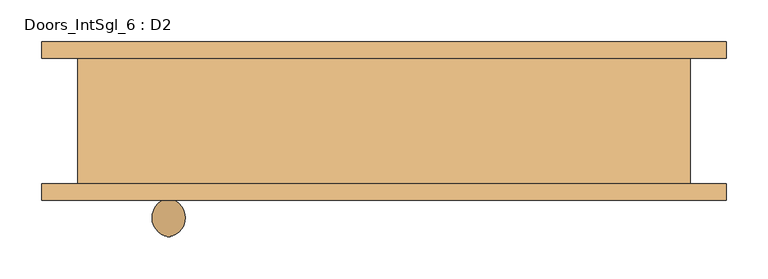
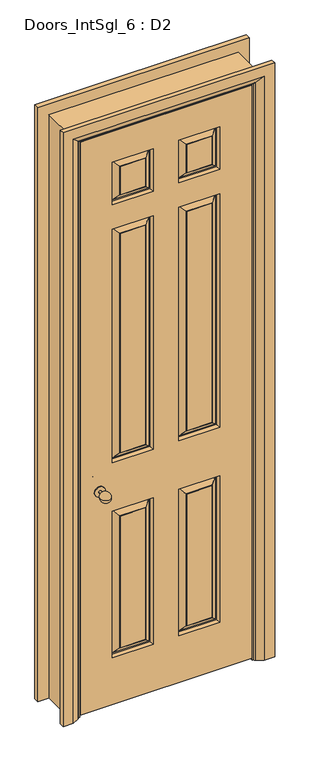
"""IFC4 building model written with IfcOpenShell, lengths in millimetres: door geometry, Doors_IntSgl_6 : D2."""

from ifc_helpers import new_model, si_unit, point, frame, origin, place, context, project, spatial, polyline, circle_curve, ellipse_curve, trimmed, outline, extrude, faceted_brep, source, transform, mapped, element, save
from ifc_brep_helpers import plane_surface, cylinder_surface, revolved_surface, advanced_brep


def doors_intsgl_6_d2_ad12cddb(model_context):
    return source(origin(), model_context, "Body", "SolidModel", [
        advanced_brep(
        [(-253.0, -18.0, 900.0), (-263.0, -18.0, 900.0), (-258.0, 26.437411, 900.0), (-253.0, -33.0, 900.0), (-263.0, -33.0, 900.0), (-278.0, -37.0, 900.0), (-238.0, -37.0, 900.0), (-278.0, -33.0, 900.0), (-238.0, -33.0, 900.0)],
        [
            (0, 1, circle_curve(frame((-258.0, -18.0, 900.0), z_axis=(0.0, 1.0, 0.0), x_axis=(-1.0, 0.0, 0.0)), 5.0)),
            (1, 2, circle_curve(frame((-254.8115138, 3.5786495, 900.0), z_axis=(0.0, 0.0, -1.0), x_axis=(0.0, -1.0, 0.0)), 23.0800654)),
            (2, 0, circle_curve(frame((-261.1884862, 3.5786495, 900.0), z_axis=(0.0, 0.0, -1.0), x_axis=(0.0, -1.0, 0.0)), 23.0800654)),
            (1, 0, circle_curve(frame((-258.0, -18.0, 900.0), z_axis=(0.0, 1.0, 0.0), x_axis=(-1.0, 0.0, 0.0)), 5.0)),
            (0, 3),
            (3, 4, circle_curve(frame((-258.0, -33.0, 900.0), z_axis=(0.0, 1.0, 0.0), x_axis=(-1.0, 0.0, 0.0)), 5.0)),
            (4, 1),
            (4, 3, circle_curve(frame((-258.0, -33.0, 900.0), z_axis=(0.0, 1.0, 0.0), x_axis=(-1.0, 0.0, 0.0)), 5.0)),
            (5, 6, circle_curve(frame((-258.0, -37.0, 900.0), z_axis=(0.0, -1.0, 0.0), x_axis=(1.0, 0.0, 0.0)), 20.0)),
            (6, 5, circle_curve(frame((-258.0, -37.0, 900.0), z_axis=(0.0, -1.0, 0.0), x_axis=(1.0, 0.0, 0.0)), 20.0)),
            (7, 8, circle_curve(frame((-258.0, -33.0, 900.0), z_axis=(0.0, 1.0, 0.0), x_axis=(1.0, 0.0, 0.0)), 20.0)),
            (8, 7, circle_curve(frame((-258.0, -33.0, 900.0), z_axis=(0.0, 1.0, 0.0), x_axis=(1.0, 0.0, 0.0)), 20.0)),
            (5, 7),
            (8, 6),
        ],
        [
            revolved_surface(trimmed(ellipse_curve(frame((-254.8115138, 3.5786495, 900.0), z_axis=(0.0, 0.0, 1.0), x_axis=(0.0, -1.0, 0.0)), 23.0800654, 23.0800654), [point((-258.0, 26.437411, 900.0))], [point((-263.0, -18.0, 900.0))], True, "CARTESIAN"), (-258.0, -33.0, 900.0), (0.0, -1.0, 0.0)),
            cylinder_surface(frame((-258.0, -33.0, 900.0), z_axis=(0.0, -1.0, 0.0), x_axis=(-1.0, 0.0, 0.0)), 5.0),
            plane_surface(frame((-238.0, -37.0, 900.0), z_axis=(0.0, -1.0, 0.0), x_axis=(0.0, 0.0, 1.0))),
            plane_surface(frame((-238.0, -33.0, 900.0), z_axis=(0.0, 1.0, 0.0), x_axis=(0.0, 0.0, -1.0))),
            cylinder_surface(frame((-258.0, -33.0, 900.0), z_axis=(0.0, -1.0, 0.0), x_axis=(1.0, 0.0, 0.0)), 20.0),
        ],
        [
            (0, [[1, 2, 3]]),
            (0, [[-2, 4, -3]]),
            (1, [[-1, 5, 6, 7]]),
            (1, [[-4, -7, 8, -5]]),
            (2, [[9, 10]]),
            (3, [[11, 12], [-6, -8]]),
            (4, [[-9, 13, -12, 14]]),
            (4, [[-10, -14, -11, -13]]),
        ],
    ),
        advanced_brep(
        [(-253.0, -94.0, 900.0), (-258.0, -138.437411, 900.0), (-263.0, -94.0, 900.0), (-263.0, -79.0, 900.0), (-253.0, -79.0, 900.0), (-278.0, -75.0, 900.0), (-238.0, -75.0, 900.0), (-278.0, -79.0, 900.0), (-238.0, -79.0, 900.0)],
        [
            (0, 1, circle_curve(frame((-261.1884862, -115.5786495, 900.0), z_axis=(0.0, 0.0, -1.0), x_axis=(0.0, 1.0, 0.0)), 23.0800654)),
            (1, 2, circle_curve(frame((-254.8115138, -115.5786495, 900.0), z_axis=(0.0, 0.0, -1.0), x_axis=(0.0, 1.0, 0.0)), 23.0800654)),
            (2, 0, circle_curve(frame((-258.0, -94.0, 900.0), z_axis=(0.0, -1.0, 0.0), x_axis=(-1.0, 0.0, 0.0)), 5.0)),
            (0, 2, circle_curve(frame((-258.0, -94.0, 900.0), z_axis=(0.0, -1.0, 0.0), x_axis=(-1.0, 0.0, 0.0)), 5.0)),
            (2, 3),
            (3, 4, circle_curve(frame((-258.0, -79.0, 900.0), z_axis=(0.0, -1.0, 0.0), x_axis=(-1.0, 0.0, 0.0)), 5.0)),
            (4, 0),
            (4, 3, circle_curve(frame((-258.0, -79.0, 900.0), z_axis=(0.0, -1.0, 0.0), x_axis=(-1.0, 0.0, 0.0)), 5.0)),
            (5, 6, circle_curve(frame((-258.0, -75.0, 900.0), z_axis=(0.0, 1.0, 0.0), x_axis=(1.0, 0.0, 0.0)), 20.0)),
            (6, 5, circle_curve(frame((-258.0, -75.0, 900.0), z_axis=(0.0, 1.0, 0.0), x_axis=(1.0, 0.0, 0.0)), 20.0)),
            (7, 8, circle_curve(frame((-258.0, -79.0, 900.0), z_axis=(0.0, -1.0, 0.0), x_axis=(1.0, 0.0, 0.0)), 20.0)),
            (8, 7, circle_curve(frame((-258.0, -79.0, 900.0), z_axis=(0.0, -1.0, 0.0), x_axis=(1.0, 0.0, 0.0)), 20.0)),
            (6, 8),
            (7, 5),
        ],
        [
            revolved_surface(trimmed(ellipse_curve(frame((-254.8115138, -115.5786495, 900.0), z_axis=(0.0, 0.0, -1.0), x_axis=(0.0, 1.0, 0.0)), 23.0800654, 23.0800654), [point((-258.0, -138.437411, 900.0))], [point((-263.0, -94.0, 900.0))], True, "CARTESIAN"), (-258.0, -79.0, 900.0), (0.0, 1.0, 0.0)),
            cylinder_surface(frame((-258.0, -79.0, 900.0), z_axis=(0.0, 1.0, 0.0), x_axis=(-1.0, 0.0, 0.0)), 5.0),
            plane_surface(frame((-238.0, -75.0, 900.0), z_axis=(0.0, 1.0, 0.0), x_axis=(0.0, 0.0, 1.0))),
            plane_surface(frame((-238.0, -79.0, 900.0), z_axis=(0.0, -1.0, 0.0), x_axis=(0.0, 0.0, -1.0))),
            cylinder_surface(frame((-258.0, -79.0, 900.0), z_axis=(0.0, 1.0, 0.0), x_axis=(1.0, 0.0, 0.0)), 20.0),
        ],
        [
            (0, [[1, 2, 3]]),
            (0, [[-1, 4, -2]]),
            (1, [[5, 6, 7, -3]]),
            (1, [[-7, 8, -5, -4]]),
            (2, [[9, 10]]),
            (3, [[11, 12], [-8, -6]]),
            (4, [[13, -11, 14, -10]]),
            (4, [[-14, -12, -13, -9]]),
        ],
    ),
        faceted_brep([(-333.0, -37.0, 2358.0), (333.0, -37.0, 2358.0), (333.0, -37.0, 8.0), (-333.0, -37.0, 8.0), (-50.0, -37.0, 800.0), (-208.0, -37.0, 800.0), (-208.0, -37.0, 200.0), (-50.0, -37.0, 200.0), (208.0, -37.0, 800.0), (50.0, -37.0, 800.0), (50.0, -37.0, 200.0), (208.0, -37.0, 200.0), (-50.0, -37.0, 1958.0), (-208.0, -37.0, 1958.0), (-208.0, -37.0, 1000.0), (-50.0, -37.0, 1000.0), (208.0, -37.0, 1958.0), (50.0, -37.0, 1958.0), (50.0, -37.0, 1000.0), (208.0, -37.0, 1000.0), (-50.0, -37.0, 2233.0), (-208.0, -37.0, 2233.0), (-208.0, -37.0, 2058.0), (-50.0, -37.0, 2058.0), (208.0, -37.0, 2233.0), (50.0, -37.0, 2233.0), (50.0, -37.0, 2058.0), (208.0, -37.0, 2058.0), (-80.0, -37.0, 230.0), (-178.0, -37.0, 230.0), (-178.0, -37.0, 770.0), (-80.0, -37.0, 770.0), (178.0, -37.0, 230.0), (80.0, -37.0, 230.0), (80.0, -37.0, 770.0), (178.0, -37.0, 770.0), (-80.0, -37.0, 1030.0), (-178.0, -37.0, 1030.0), (-178.0, -37.0, 1928.0), (-80.0, -37.0, 1928.0), (178.0, -37.0, 1030.0), (80.0, -37.0, 1030.0), (80.0, -37.0, 1928.0), (178.0, -37.0, 1928.0), (-80.0, -37.0, 2088.0), (-178.0, -37.0, 2088.0), (-178.0, -37.0, 2203.0), (-80.0, -37.0, 2203.0), (178.0, -37.0, 2088.0), (80.0, -37.0, 2088.0), (80.0, -37.0, 2203.0), (178.0, -37.0, 2203.0), (-333.0, -75.0, 2358.0), (-333.0, -75.0, 8.0), (333.0, -75.0, 8.0), (333.0, -75.0, 2358.0), (50.0, -75.0, 800.0), (208.0, -75.0, 800.0), (208.0, -75.0, 200.0), (50.0, -75.0, 200.0), (-208.0, -75.0, 800.0), (-50.0, -75.0, 800.0), (-50.0, -75.0, 200.0), (-208.0, -75.0, 200.0), (50.0, -75.0, 1958.0), (208.0, -75.0, 1958.0), (208.0, -75.0, 1000.0), (50.0, -75.0, 1000.0), (-208.0, -75.0, 1958.0), (-50.0, -75.0, 1958.0), (-50.0, -75.0, 1000.0), (-208.0, -75.0, 1000.0), (50.0, -75.0, 2233.0), (208.0, -75.0, 2233.0), (208.0, -75.0, 2058.0), (50.0, -75.0, 2058.0), (-208.0, -75.0, 2233.0), (-50.0, -75.0, 2233.0), (-50.0, -75.0, 2058.0), (-208.0, -75.0, 2058.0), (80.0, -75.0, 230.0), (178.0, -75.0, 230.0), (178.0, -75.0, 770.0), (80.0, -75.0, 770.0), (-178.0, -75.0, 230.0), (-80.0, -75.0, 230.0), (-80.0, -75.0, 770.0), (-178.0, -75.0, 770.0), (80.0, -75.0, 1030.0), (178.0, -75.0, 1030.0), (178.0, -75.0, 1928.0), (80.0, -75.0, 1928.0), (-178.0, -75.0, 1030.0), (-80.0, -75.0, 1030.0), (-80.0, -75.0, 1928.0), (-178.0, -75.0, 1928.0), (80.0, -75.0, 2088.0), (178.0, -75.0, 2088.0), (178.0, -75.0, 2203.0), (80.0, -75.0, 2203.0), (-178.0, -75.0, 2088.0), (-80.0, -75.0, 2088.0), (-80.0, -75.0, 2203.0), (-178.0, -75.0, 2203.0), (80.0, -74.0, 230.0), (80.0, -74.0, 770.0), (58.0, -60.0, 208.0), (78.0, -74.0, 228.0), (78.0, -74.0, 772.0), (58.0, -60.0, 792.0), (53.0, -60.0, 203.0), (53.0, -60.0, 797.0), (178.0, -74.0, 770.0), (180.0, -74.0, 772.0), (200.0, -60.0, 792.0), (205.0, -60.0, 797.0), (178.0, -74.0, 230.0), (180.0, -74.0, 228.0), (200.0, -60.0, 208.0), (205.0, -60.0, 203.0), (-178.0, -74.0, 230.0), (-178.0, -74.0, 770.0), (-200.0, -60.0, 208.0), (-180.0, -74.0, 228.0), (-180.0, -74.0, 772.0), (-200.0, -60.0, 792.0), (-205.0, -60.0, 203.0), (-205.0, -60.0, 797.0), (-80.0, -74.0, 770.0), (-78.0, -74.0, 772.0), (-58.0, -60.0, 792.0), (-53.0, -60.0, 797.0), (-80.0, -74.0, 230.0), (-78.0, -74.0, 228.0), (-58.0, -60.0, 208.0), (-53.0, -60.0, 203.0), (80.0, -74.0, 1030.0), (80.0, -74.0, 1928.0), (58.0, -60.0, 1008.0), (78.0, -74.0, 1028.0), (78.0, -74.0, 1930.0), (58.0, -60.0, 1950.0), (53.0, -60.0, 1003.0), (53.0, -60.0, 1955.0), (178.0, -74.0, 1928.0), (180.0, -74.0, 1930.0), (200.0, -60.0, 1950.0), (205.0, -60.0, 1955.0), (178.0, -74.0, 1030.0), (180.0, -74.0, 1028.0), (200.0, -60.0, 1008.0), (205.0, -60.0, 1003.0), (-178.0, -74.0, 1030.0), (-178.0, -74.0, 1928.0), (-200.0, -60.0, 1008.0), (-180.0, -74.0, 1028.0), (-180.0, -74.0, 1930.0), (-200.0, -60.0, 1950.0), (-205.0, -60.0, 1003.0), (-205.0, -60.0, 1955.0), (-80.0, -74.0, 1928.0), (-78.0, -74.0, 1930.0), (-58.0, -60.0, 1950.0), (-53.0, -60.0, 1955.0), (-80.0, -74.0, 1030.0), (-78.0, -74.0, 1028.0), (-58.0, -60.0, 1008.0), (-53.0, -60.0, 1003.0), (80.0, -74.0, 2088.0), (80.0, -74.0, 2203.0), (58.0, -60.0, 2066.0), (78.0, -74.0, 2086.0), (78.0, -74.0, 2205.0), (58.0, -60.0, 2225.0), (53.0, -60.0, 2061.0), (53.0, -60.0, 2230.0), (178.0, -74.0, 2203.0), (180.0, -74.0, 2205.0), (200.0, -60.0, 2225.0), (205.0, -60.0, 2230.0), (178.0, -74.0, 2088.0), (180.0, -74.0, 2086.0), (200.0, -60.0, 2066.0), (205.0, -60.0, 2061.0), (-178.0, -74.0, 2088.0), (-178.0, -74.0, 2203.0), (-200.0, -60.0, 2066.0), (-180.0, -74.0, 2086.0), (-180.0, -74.0, 2205.0), (-200.0, -60.0, 2225.0), (-205.0, -60.0, 2061.0), (-205.0, -60.0, 2230.0), (-80.0, -74.0, 2203.0), (-78.0, -74.0, 2205.0), (-58.0, -60.0, 2225.0), (-53.0, -60.0, 2230.0), (-80.0, -74.0, 2088.0), (-78.0, -74.0, 2086.0), (-58.0, -60.0, 2066.0), (-53.0, -60.0, 2061.0), (-80.0, -38.0, 230.0), (-80.0, -38.0, 770.0), (-58.0, -52.0, 208.0), (-78.0, -38.0, 228.0), (-78.0, -38.0, 772.0), (-58.0, -52.0, 792.0), (-53.0, -52.0, 203.0), (-53.0, -52.0, 797.0), (-178.0, -38.0, 770.0), (-180.0, -38.0, 772.0), (-200.0, -52.0, 792.0), (-205.0, -52.0, 797.0), (-178.0, -38.0, 230.0), (-180.0, -38.0, 228.0), (-200.0, -52.0, 208.0), (-205.0, -52.0, 203.0), (178.0, -38.0, 230.0), (178.0, -38.0, 770.0), (200.0, -52.0, 208.0), (180.0, -38.0, 228.0), (180.0, -38.0, 772.0), (200.0, -52.0, 792.0), (205.0, -52.0, 203.0), (205.0, -52.0, 797.0), (80.0, -38.0, 770.0), (78.0, -38.0, 772.0), (58.0, -52.0, 792.0), (53.0, -52.0, 797.0), (80.0, -38.0, 230.0), (78.0, -38.0, 228.0), (58.0, -52.0, 208.0), (53.0, -52.0, 203.0), (-80.0, -38.0, 1030.0), (-80.0, -38.0, 1928.0), (-58.0, -52.0, 1008.0), (-78.0, -38.0, 1028.0), (-78.0, -38.0, 1930.0), (-58.0, -52.0, 1950.0), (-53.0, -52.0, 1003.0), (-53.0, -52.0, 1955.0), (-178.0, -38.0, 1928.0), (-180.0, -38.0, 1930.0), (-200.0, -52.0, 1950.0), (-205.0, -52.0, 1955.0), (-178.0, -38.0, 1030.0), (-180.0, -38.0, 1028.0), (-200.0, -52.0, 1008.0), (-205.0, -52.0, 1003.0), (178.0, -38.0, 1030.0), (178.0, -38.0, 1928.0), (200.0, -52.0, 1008.0), (180.0, -38.0, 1028.0), (180.0, -38.0, 1930.0), (200.0, -52.0, 1950.0), (205.0, -52.0, 1003.0), (205.0, -52.0, 1955.0), (80.0, -38.0, 1928.0), (78.0, -38.0, 1930.0), (58.0, -52.0, 1950.0), (53.0, -52.0, 1955.0), (80.0, -38.0, 1030.0), (78.0, -38.0, 1028.0), (58.0, -52.0, 1008.0), (53.0, -52.0, 1003.0), (-80.0, -38.0, 2088.0), (-80.0, -38.0, 2203.0), (-58.0, -52.0, 2066.0), (-78.0, -38.0, 2086.0), (-78.0, -38.0, 2205.0), (-58.0, -52.0, 2225.0), (-53.0, -52.0, 2061.0), (-53.0, -52.0, 2230.0), (-178.0, -38.0, 2203.0), (-180.0, -38.0, 2205.0), (-200.0, -52.0, 2225.0), (-205.0, -52.0, 2230.0), (-178.0, -38.0, 2088.0), (-180.0, -38.0, 2086.0), (-200.0, -52.0, 2066.0), (-205.0, -52.0, 2061.0), (178.0, -38.0, 2088.0), (178.0, -38.0, 2203.0), (200.0, -52.0, 2066.0), (180.0, -38.0, 2086.0), (180.0, -38.0, 2205.0), (200.0, -52.0, 2225.0), (205.0, -52.0, 2061.0), (205.0, -52.0, 2230.0), (80.0, -38.0, 2203.0), (78.0, -38.0, 2205.0), (58.0, -52.0, 2225.0), (53.0, -52.0, 2230.0), (80.0, -38.0, 2088.0), (78.0, -38.0, 2086.0), (58.0, -52.0, 2066.0), (53.0, -52.0, 2061.0)], [[[0, 1, 2, 3], [4, 5, 6, 7], [8, 9, 10, 11], [12, 13, 14, 15], [16, 17, 18, 19], [20, 21, 22, 23], [24, 25, 26, 27]], [[28, 29, 30, 31]], [[32, 33, 34, 35]], [[36, 37, 38, 39]], [[40, 41, 42, 43]], [[44, 45, 46, 47]], [[48, 49, 50, 51]], [[52, 53, 54, 55], [56, 57, 58, 59], [60, 61, 62, 63], [64, 65, 66, 67], [68, 69, 70, 71], [72, 73, 74, 75], [76, 77, 78, 79]], [[80, 81, 82, 83]], [[84, 85, 86, 87]], [[88, 89, 90, 91]], [[92, 93, 94, 95]], [[96, 97, 98, 99]], [[100, 101, 102, 103]], [[3, 53, 52, 0]], [[2, 54, 53, 3]], [[1, 55, 54, 2]], [[0, 52, 55, 1]], [[104, 80, 83, 105]], [[106, 107, 108, 109]], [[56, 59, 110, 111]], [[83, 82, 112, 105]], [[108, 113, 114, 109]], [[111, 115, 57, 56]], [[82, 81, 116, 112]], [[113, 117, 118, 114]], [[115, 119, 58, 57]], [[104, 116, 81, 80]], [[107, 117, 113, 108], [105, 112, 116, 104]], [[106, 118, 117, 107]], [[110, 119, 115, 111], [109, 114, 118, 106]], [[59, 58, 119, 110]], [[120, 84, 87, 121]], [[122, 123, 124, 125]], [[60, 63, 126, 127]], [[87, 86, 128, 121]], [[124, 129, 130, 125]], [[127, 131, 61, 60]], [[86, 85, 132, 128]], [[129, 133, 134, 130]], [[131, 135, 62, 61]], [[120, 132, 85, 84]], [[123, 133, 129, 124], [121, 128, 132, 120]], [[122, 134, 133, 123]], [[126, 135, 131, 127], [125, 130, 134, 122]], [[63, 62, 135, 126]], [[136, 88, 91, 137]], [[138, 139, 140, 141]], [[64, 67, 142, 143]], [[91, 90, 144, 137]], [[140, 145, 146, 141]], [[143, 147, 65, 64]], [[90, 89, 148, 144]], [[145, 149, 150, 146]], [[147, 151, 66, 65]], [[136, 148, 89, 88]], [[139, 149, 145, 140], [137, 144, 148, 136]], [[138, 150, 149, 139]], [[142, 151, 147, 143], [141, 146, 150, 138]], [[67, 66, 151, 142]], [[152, 92, 95, 153]], [[154, 155, 156, 157]], [[68, 71, 158, 159]], [[95, 94, 160, 153]], [[156, 161, 162, 157]], [[159, 163, 69, 68]], [[94, 93, 164, 160]], [[161, 165, 166, 162]], [[163, 167, 70, 69]], [[152, 164, 93, 92]], [[155, 165, 161, 156], [153, 160, 164, 152]], [[154, 166, 165, 155]], [[158, 167, 163, 159], [157, 162, 166, 154]], [[71, 70, 167, 158]], [[168, 96, 99, 169]], [[170, 171, 172, 173]], [[72, 75, 174, 175]], [[99, 98, 176, 169]], [[172, 177, 178, 173]], [[175, 179, 73, 72]], [[98, 97, 180, 176]], [[177, 181, 182, 178]], [[179, 183, 74, 73]], [[168, 180, 97, 96]], [[171, 181, 177, 172], [169, 176, 180, 168]], [[170, 182, 181, 171]], [[174, 183, 179, 175], [173, 178, 182, 170]], [[75, 74, 183, 174]], [[184, 100, 103, 185]], [[186, 187, 188, 189]], [[76, 79, 190, 191]], [[103, 102, 192, 185]], [[188, 193, 194, 189]], [[191, 195, 77, 76]], [[102, 101, 196, 192]], [[193, 197, 198, 194]], [[195, 199, 78, 77]], [[184, 196, 101, 100]], [[187, 197, 193, 188], [185, 192, 196, 184]], [[186, 198, 197, 187]], [[190, 199, 195, 191], [189, 194, 198, 186]], [[79, 78, 199, 190]], [[200, 28, 31, 201]], [[202, 203, 204, 205]], [[4, 7, 206, 207]], [[31, 30, 208, 201]], [[204, 209, 210, 205]], [[207, 211, 5, 4]], [[30, 29, 212, 208]], [[209, 213, 214, 210]], [[211, 215, 6, 5]], [[200, 212, 29, 28]], [[203, 213, 209, 204], [201, 208, 212, 200]], [[202, 214, 213, 203]], [[206, 215, 211, 207], [205, 210, 214, 202]], [[7, 6, 215, 206]], [[216, 32, 35, 217]], [[218, 219, 220, 221]], [[8, 11, 222, 223]], [[35, 34, 224, 217]], [[220, 225, 226, 221]], [[223, 227, 9, 8]], [[34, 33, 228, 224]], [[225, 229, 230, 226]], [[227, 231, 10, 9]], [[216, 228, 33, 32]], [[219, 229, 225, 220], [217, 224, 228, 216]], [[218, 230, 229, 219]], [[222, 231, 227, 223], [221, 226, 230, 218]], [[11, 10, 231, 222]], [[232, 36, 39, 233]], [[234, 235, 236, 237]], [[12, 15, 238, 239]], [[39, 38, 240, 233]], [[236, 241, 242, 237]], [[239, 243, 13, 12]], [[38, 37, 244, 240]], [[241, 245, 246, 242]], [[243, 247, 14, 13]], [[232, 244, 37, 36]], [[235, 245, 241, 236], [233, 240, 244, 232]], [[234, 246, 245, 235]], [[238, 247, 243, 239], [237, 242, 246, 234]], [[15, 14, 247, 238]], [[248, 40, 43, 249]], [[250, 251, 252, 253]], [[16, 19, 254, 255]], [[43, 42, 256, 249]], [[252, 257, 258, 253]], [[255, 259, 17, 16]], [[42, 41, 260, 256]], [[257, 261, 262, 258]], [[259, 263, 18, 17]], [[248, 260, 41, 40]], [[251, 261, 257, 252], [249, 256, 260, 248]], [[250, 262, 261, 251]], [[254, 263, 259, 255], [253, 258, 262, 250]], [[19, 18, 263, 254]], [[264, 44, 47, 265]], [[266, 267, 268, 269]], [[20, 23, 270, 271]], [[47, 46, 272, 265]], [[268, 273, 274, 269]], [[271, 275, 21, 20]], [[46, 45, 276, 272]], [[273, 277, 278, 274]], [[275, 279, 22, 21]], [[264, 276, 45, 44]], [[267, 277, 273, 268], [265, 272, 276, 264]], [[266, 278, 277, 267]], [[270, 279, 275, 271], [269, 274, 278, 266]], [[23, 22, 279, 270]], [[280, 48, 51, 281]], [[282, 283, 284, 285]], [[24, 27, 286, 287]], [[51, 50, 288, 281]], [[284, 289, 290, 285]], [[287, 291, 25, 24]], [[50, 49, 292, 288]], [[289, 293, 294, 290]], [[291, 295, 26, 25]], [[280, 292, 49, 48]], [[283, 293, 289, 284], [281, 288, 292, 280]], [[282, 294, 293, 283]], [[286, 295, 291, 287], [285, 290, 294, 282]], [[27, 26, 295, 286]]]),
        faceted_brep([(-335.0, -75.0, 0.0), (-367.0, -75.0, 0.0), (-367.0, 75.0, 0.0), (-335.0, 75.0, 0.0), (-335.0, 75.0, 2360.0), (-335.0, -75.0, 2360.0), (-367.0, 75.0, 2392.0), (-367.0, -75.0, 2392.0), (335.0, -75.0, 0.0), (335.0, 75.0, 0.0), (367.0, 75.0, 0.0), (367.0, -75.0, 0.0), (335.0, -75.0, 2360.0), (367.0, -75.0, 2392.0), (367.0, 75.0, 2392.0), (335.0, 75.0, 2360.0)], [[[0, 1, 2, 3]], [[3, 4, 5, 0]], [[2, 6, 4, 3]], [[1, 7, 6, 2]], [[0, 5, 7, 1]], [[8, 9, 10, 11]], [[12, 8, 11, 13]], [[13, 11, 10, 14]], [[14, 10, 9, 15]], [[15, 9, 8, 12]], [[4, 15, 12, 5]], [[6, 14, 15, 4]], [[7, 13, 14, 6]], [[5, 12, 13, 7]]]),
        extrude(outline(polyline([(0.0, -316.0), (2341.0, -316.0), (2341.0, 316.0), (0.0, 316.0), (0.0, 335.0), (2360.0, 335.0), (2360.0, -335.0), (0.0, -335.0), (0.0, -316.0)])), frame((0.0, -35.0, 0.0), z_axis=(0.0, 1.0, 0.0), x_axis=(0.0, 0.0, 1.0)), (0.0, 0.0, 1.0), 32.0),
        advanced_brep(
        [(-410.0, 95.0, 0.0), (-370.0, 95.0, 0.0), (-344.0, 81.0, 0.0), (-340.0, 75.0, 0.0), (-410.0, 75.0, 0.0), (-410.0, 75.0, 2435.0), (-410.0, 95.0, 2435.0), (-340.0, 75.0, 2365.0), (340.0, 75.0, 2365.0), (340.0, 75.0, 0.0), (410.0, 75.0, 0.0), (410.0, 75.0, 2435.0), (-344.0, 81.0, 2369.0), (-370.0, 95.0, 2395.0), (410.0, 95.0, 2435.0), (410.0, 95.0, 0.0), (370.0, 95.0, 0.0), (370.0, 95.0, 2395.0), (344.0, 81.0, 0.0), (344.0, 81.0, 2369.0)],
        [
            (0, 1),
            (1, 2),
            (2, 3, circle_curve(frame((-348.0, 74.0, 0.0), z_axis=(0.0, 0.0, -1.0), x_axis=(-1.0, 0.0, 0.0)), 8.0622577)),
            (3, 4),
            (4, 0),
            (4, 5),
            (5, 6),
            (6, 0),
            (3, 7),
            (7, 8),
            (8, 9),
            (9, 10),
            (10, 11),
            (11, 5),
            (2, 12),
            (12, 7, ellipse_curve(frame((-348.0, 74.0, 2373.0), z_axis=(-0.7071067811865475, 0.0, -0.7071067811865475), x_axis=(0.7071067811865474, 0.0, -0.7071067811865476)), 11.4017543, 8.0622577)),
            (1, 13),
            (13, 12),
            (6, 14),
            (14, 15),
            (15, 16),
            (16, 17),
            (17, 13),
            (10, 15),
            (14, 11),
            (9, 18, circle_curve(frame((348.0, 74.0, 0.0), z_axis=(0.0, 0.0, -1.0), x_axis=(1.0, 0.0, 0.0)), 8.0622577)),
            (18, 16),
            (19, 18),
            (8, 19, ellipse_curve(frame((348.0, 74.0, 2373.0), z_axis=(0.7071067811865475, 0.0, -0.7071067811865475), x_axis=(0.7071067811865474, 0.0, 0.7071067811865476)), 11.4017543, 8.0622577)),
            (19, 17),
            (12, 19),
        ],
        [
            plane_surface(frame((-340.0, 75.0, 0.0), z_axis=(0.0, 0.0, -1.0), x_axis=(0.0, 1.0, 0.0))),
            plane_surface(frame((-410.0, 95.0, 0.0), z_axis=(-1.0, 0.0, 0.0), x_axis=(0.0, 0.0, 1.0))),
            plane_surface(frame((-410.0, 75.0, 0.0), z_axis=(0.0, -1.0, 0.0), x_axis=(0.0, 0.0, 1.0))),
            cylinder_surface(frame((-348.0, 74.0, 0.0), z_axis=(0.0, 0.0, -1.0), x_axis=(-1.0, 0.0, 0.0)), 8.0622577),
            plane_surface(frame((-344.0, 81.0, 0.0), z_axis=(0.4740998230350183, 0.8804710999221749, 0.0), x_axis=(0.0, 0.0, 1.0))),
            plane_surface(frame((-370.0, 95.0, 0.0), z_axis=(0.0, 1.0, 0.0), x_axis=(0.0, 0.0, 1.0))),
            plane_surface(frame((410.0, 95.0, 2435.0), z_axis=(1.0, 0.0, 0.0), x_axis=(0.0, 0.0, -1.0))),
            plane_surface(frame((340.0, 75.0, 0.0), z_axis=(0.0, 0.0, -1.0), x_axis=(0.0, 1.0, 0.0))),
            cylinder_surface(frame((348.0, 74.0, 2365.0), z_axis=(0.0, 0.0, 1.0), x_axis=(1.0, 0.0, 0.0)), 8.0622577),
            plane_surface(frame((344.0, 81.0, 2369.0), z_axis=(-0.4740998230350183, 0.8804710999221749, 0.0), x_axis=(0.0, 0.0, -1.0))),
            plane_surface(frame((-410.0, 95.0, 2435.0), z_axis=(0.0, 0.0, 1.0), x_axis=(1.0, 0.0, 0.0))),
            cylinder_surface(frame((-340.0, 74.0, 2373.0), z_axis=(-1.0, 0.0, 0.0), x_axis=(0.0, 0.0, 1.0)), 8.0622577),
            plane_surface(frame((-344.0, 81.0, 2369.0), z_axis=(0.0, 0.8804710999221749, -0.4740998230350183), x_axis=(1.0, 0.0, 0.0))),
        ],
        [
            (0, [[1, 2, 3, 4, 5]]),
            (1, [[6, 7, 8, -5]]),
            (2, [[9, 10, 11, 12, 13, 14, -6, -4]]),
            (3, [[15, 16, -9, -3]]),
            (4, [[17, 18, -15, -2]]),
            (5, [[-8, 19, 20, 21, 22, 23, -17, -1]]),
            (6, [[-13, 24, -20, 25]]),
            (7, [[-24, -12, 26, 27, -21]]),
            (8, [[28, -26, -11, 29]]),
            (9, [[-22, -27, -28, 30]]),
            (10, [[-14, -25, -19, -7]]),
            (11, [[31, -29, -10, -16]]),
            (12, [[-23, -30, -31, -18]]),
        ],
    ),
        advanced_brep(
        [(410.0, -95.0, 0.0), (370.0, -95.0, 0.0), (344.0, -81.0, 0.0), (340.0, -75.0, 0.0), (410.0, -75.0, 0.0), (410.0, -75.0, 2435.0), (410.0, -95.0, 2435.0), (340.0, -75.0, 2365.0), (-340.0, -75.0, 2365.0), (-340.0, -75.0, 0.0), (-410.0, -75.0, 0.0), (-410.0, -75.0, 2435.0), (344.0, -81.0, 2369.0), (370.0, -95.0, 2395.0), (-410.0, -95.0, 2435.0), (-410.0, -95.0, 0.0), (-370.0, -95.0, 0.0), (-370.0, -95.0, 2395.0), (-344.0, -81.0, 0.0), (-344.0, -81.0, 2369.0)],
        [
            (0, 1),
            (1, 2),
            (2, 3, circle_curve(frame((348.0, -74.0, 0.0), z_axis=(0.0, 0.0, -1.0), x_axis=(1.0, 0.0, 0.0)), 8.0622577)),
            (3, 4),
            (4, 0),
            (4, 5),
            (5, 6),
            (6, 0),
            (3, 7),
            (7, 8),
            (8, 9),
            (9, 10),
            (10, 11),
            (11, 5),
            (2, 12),
            (12, 7, ellipse_curve(frame((348.0, -74.0, 2373.0), z_axis=(0.7071067811865475, 0.0, -0.7071067811865475), x_axis=(-0.7071067811865474, 0.0, -0.7071067811865476)), 11.4017543, 8.0622577)),
            (1, 13),
            (13, 12),
            (6, 14),
            (14, 15),
            (15, 16),
            (16, 17),
            (17, 13),
            (10, 15),
            (14, 11),
            (9, 18, circle_curve(frame((-348.0, -74.0, 0.0), z_axis=(0.0, 0.0, -1.0), x_axis=(-1.0, 0.0, 0.0)), 8.0622577)),
            (18, 16),
            (19, 18),
            (8, 19, ellipse_curve(frame((-348.0, -74.0, 2373.0), z_axis=(-0.7071067811865475, 0.0, -0.7071067811865475), x_axis=(-0.7071067811865474, 0.0, 0.7071067811865476)), 11.4017543, 8.0622577)),
            (19, 17),
            (12, 19),
        ],
        [
            plane_surface(frame((340.0, -75.0, 0.0), z_axis=(0.0, 0.0, -1.0), x_axis=(0.0, -1.0, 0.0))),
            plane_surface(frame((410.0, -95.0, 0.0), z_axis=(1.0, 0.0, 0.0), x_axis=(0.0, 0.0, 1.0))),
            plane_surface(frame((410.0, -75.0, 0.0), z_axis=(0.0, 1.0, 0.0), x_axis=(0.0, 0.0, 1.0))),
            cylinder_surface(frame((348.0, -74.0, 0.0), z_axis=(0.0, 0.0, -1.0), x_axis=(1.0, 0.0, 0.0)), 8.0622577),
            plane_surface(frame((344.0, -81.0, 0.0), z_axis=(-0.4740998230350183, -0.8804710999221749, 0.0), x_axis=(0.0, 0.0, 1.0))),
            plane_surface(frame((370.0, -95.0, 0.0), z_axis=(0.0, -1.0, 0.0), x_axis=(0.0, 0.0, 1.0))),
            plane_surface(frame((-410.0, -95.0, 2435.0), z_axis=(-1.0, 0.0, 0.0), x_axis=(0.0, 0.0, -1.0))),
            plane_surface(frame((-340.0, -75.0, 0.0), z_axis=(0.0, 0.0, -1.0), x_axis=(0.0, -1.0, 0.0))),
            cylinder_surface(frame((-348.0, -74.0, 2365.0), z_axis=(0.0, 0.0, 1.0), x_axis=(-1.0, 0.0, 0.0)), 8.0622577),
            plane_surface(frame((-344.0, -81.0, 2369.0), z_axis=(0.4740998230350183, -0.8804710999221749, 0.0), x_axis=(0.0, 0.0, -1.0))),
            plane_surface(frame((410.0, -95.0, 2435.0), z_axis=(0.0, 0.0, 1.0), x_axis=(-1.0, 0.0, 0.0))),
            cylinder_surface(frame((340.0, -74.0, 2373.0), z_axis=(1.0, 0.0, 0.0), x_axis=(0.0, 0.0, 1.0)), 8.0622577),
            plane_surface(frame((344.0, -81.0, 2369.0), z_axis=(0.0, -0.8804710999221749, -0.4740998230350183), x_axis=(-1.0, 0.0, 0.0))),
        ],
        [
            (0, [[1, 2, 3, 4, 5]]),
            (1, [[6, 7, 8, -5]]),
            (2, [[9, 10, 11, 12, 13, 14, -6, -4]]),
            (3, [[15, 16, -9, -3]]),
            (4, [[17, 18, -15, -2]]),
            (5, [[-8, 19, 20, 21, 22, 23, -17, -1]]),
            (6, [[-13, 24, -20, 25]]),
            (7, [[-24, -12, 26, 27, -21]]),
            (8, [[28, -26, -11, 29]]),
            (9, [[-22, -27, -28, 30]]),
            (10, [[-14, -25, -19, -7]]),
            (11, [[31, -29, -10, -16]]),
            (12, [[-23, -30, -31, -18]]),
        ],
    ),
    ])


if __name__ == "__main__":
    model = new_model("IFC4")
    model_context = context("Model", 3, world=origin())
    ifc_project = project(units=[si_unit("LENGTHUNIT", "METRE", prefix="MILLI")], contexts=[model_context])
    site = spatial("IfcSite", under=ifc_project)
    building = spatial("IfcBuilding", under=site)
    placement = place(None, origin())
    doors_intsgl_6_d2_shape = doors_intsgl_6_d2_ad12cddb(model_context)
    element("IfcDoor", 1, ObjectType="Doors_IntSgl_6 : D2", at=placement, inside=building, context=model_context, shape_type="MappedRepresentation", body=[
        mapped(doors_intsgl_6_d2_shape, transform((0.0, 0.0, 0.0), x_axis=(1.0, 0.0, 0.0), y_axis=(0.0, 1.0, 0.0), z_axis=(0.0, 0.0, 1.0))),
    ])
    save(model, "model.ifc")

# Revit data of these elements
# Type "Doors_IntSgl_6 : D2"
#   Type Mark = "50"
#   Type Comments = "Internal Single"
#   Operation = "SingleSwingRight"
#   Construction Type Id = "MDOOR"
#   Manufacturer = "Revit"
#   Keynote = "L20"
#   Description = "Internal Single Door"
#   Analytic Construction = "Metal"
#   UnderCut = 8 mm
#   Tolerance = 2 mm
#   Thickness = 38 mm
#   Structural Tolerance = 8 mm
#   StopDepth = 32 mm
#   Stop Thickness = 19 mm
#   Stile Top Rail = 125 mm
#   Stile Shutting = 125 mm
#   Stile Muntin Rail = 100 mm
#   Stile Lock Rail = 200 mm
#   Stile Intermediate/Frieze = 100 mm
#   Stile Hanging = 125 mm
#   Stile Bottom Rail = 200 mm
#   Rough Width = 750 mm
#   Rough Height = 2400 mm
#   Height to Top Lock Rail = 1000 mm
#   Heat Transfer Coefficient (U) = 3.7021 W/(m²·K)
#   Handle Z Distance = 900 mm
#   Handle X Distance = 75 mm
#   Frame Thickness = 32 mm
#   Door Panel Width = 666 mm
#   Height = 2400 mm
#   Width = 750 mm
#   Door Panel Thickness = 38 mm
#   Door Panel Offset = 0 mm
#   Door Panel Height = 2350 mm
#   Architrave Setback = 5 mm
#   Vis - Ironmongery = yes
#   Define Thermal Properties by = 1
#   Material Ironmongery = Door - Handle
#   Material Frame = Door - Frame/Mullion
#   Material Door = Door - Panel
#   Material Architrave = Door - Architrave
#   Visual Light Transmittance = 0
#   Solar Heat Gain Coefficient = 0
#   Function = (empty or 0)
#   Wall Closure = (empty or 0)
# Element 1 (IfcDoor, "Doors_IntSgl_6 : D2")
#   Materials on its faces: "Door - Panel", "Door - Architrave", "Door - Frame/Mullion", "Door - Handle"
# Materials
#   "Door - Handle": colour RGB 247 247 247, transparency 0
#   "Door - Frame/Mullion": class "Wood", colour RGB 212 179 113, transparency 0
#   "Door - Panel": class "Wood", colour RGB 154 90 5, transparency 0
#   "Door - Architrave": class "Wood", colour RGB 154 90 5, transparency 0
